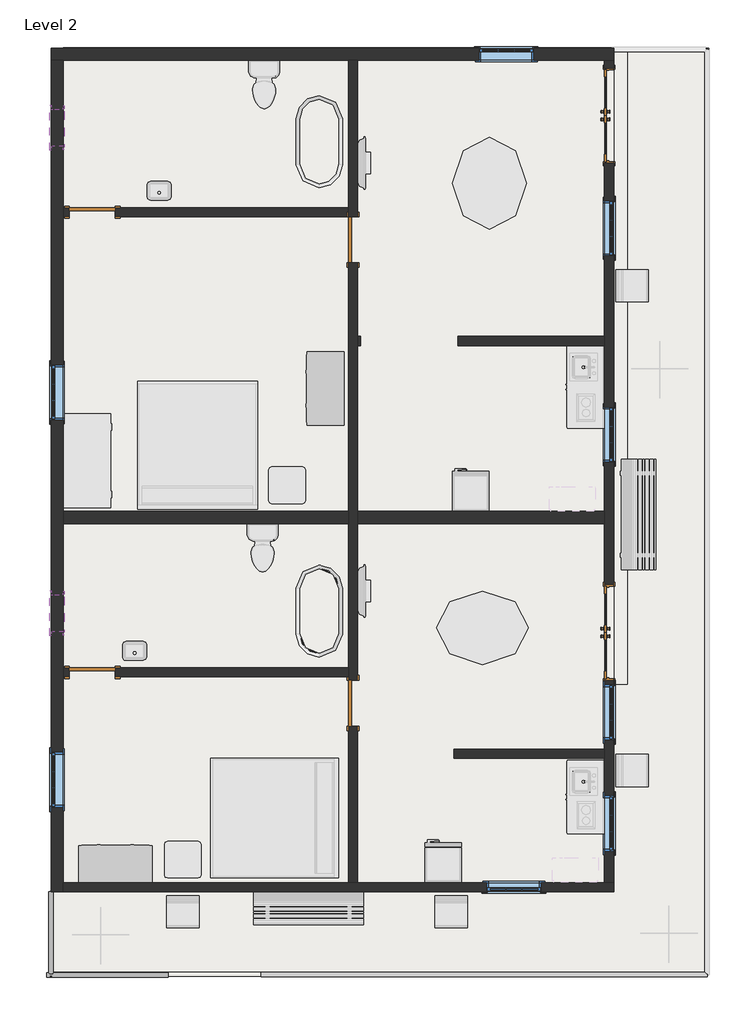
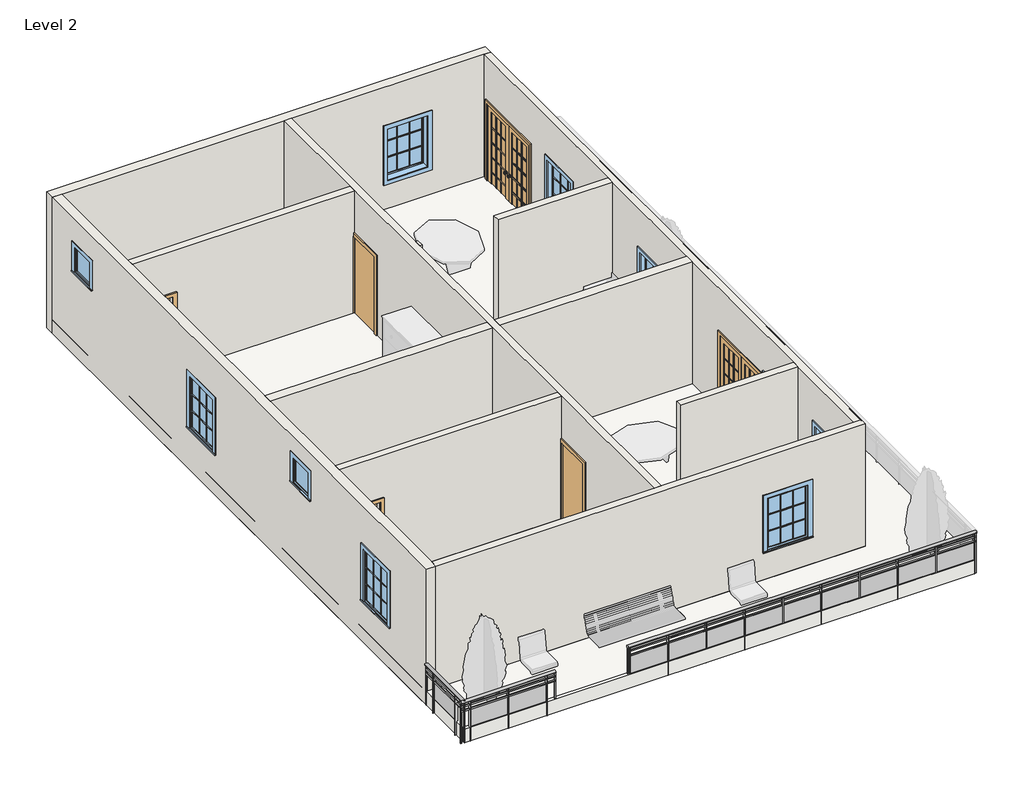
# One storey, part 1 of 2: 12 walls, 10 windows, 7 roofs, 6 doors, 3 railings.
"""IFC4 building model written with IfcOpenShell, lengths in millimetres."""

from ifc_helpers import new_model, si_unit, point, frame, origin, place, context, project, spatial, polyline, ellipse_curve, trimmed, outline, extrude, faceted_brep, transform, mapped, element, save
from ifc_brep_helpers import plane_surface, extruded_surface, advanced_brep
from components import door_31a77bde, door_255cab33, door_059fdd7e, window_29c06734, window_5c190c7e, window_e41d21a6

model = new_model("IFC4")

# Units and contexts
model_context = context("Model", 3, world=origin())
ifc_project = project(units=[si_unit("LENGTHUNIT", "METRE", prefix="MILLI")], contexts=[model_context])

# Site, building, storey
site = spatial("IfcSite", under=ifc_project)
building = spatial("IfcBuilding", under=site)
storey = spatial("IfcBuildingStorey", under=building, Name="Level 2", Elevation=3048.0)

# Doors
placement = place(None, origin())
door_shape = door_31a77bde(model_context)
element("IfcDoor", 1, ObjectType="Door-Interior-Double-Full Glass-Wood : 60\" x 80\"", at=placement, inside=storey, context=model_context, shape_type="MappedRepresentation", body=[
    mapped(door_shape, transform((230.0079734, 3216.1923354, 3048.0), x_axis=(0.0, 1.0, 0.0), y_axis=(-1.0, 0.0, 0.0), z_axis=(0.0, 0.0, 1.0))),
])
element("IfcDoor", 2, ObjectType="Door-Interior-Double-Full Glass-Wood : 60\" x 80\"", at=placement, inside=storey, context=model_context, shape_type="MappedRepresentation", body=[
    mapped(door_shape, transform((230.0079734, 11775.9923354, 3048.0), x_axis=(0.0, 1.0, 0.0), y_axis=(-1.0, 0.0, 0.0), z_axis=(0.0, 0.0, 1.0))),
])
door_2_shape = door_255cab33(model_context)
element("IfcDoor", 3, ObjectType="Single-Flush : 30\" x 80\"", at=placement, inside=storey, context=model_context, shape_type="MappedRepresentation", body=[
    mapped(door_2_shape, transform((-8326.6170266, 10175.7923354, 3048.0), x_axis=(-1.0, 0.0, 0.0), y_axis=(0.0, -1.0, 0.0), z_axis=(0.0, 0.0, 1.0))),
])
element("IfcDoor", 4, ObjectType="Single-Flush : 30\" x 80\"", at=placement, inside=storey, context=model_context, shape_type="MappedRepresentation", body=[
    mapped(door_2_shape, transform((-8326.6170266, 2555.7923354, 3048.0), x_axis=(-1.0, 0.0, 0.0), y_axis=(0.0, -1.0, 0.0), z_axis=(0.0, 0.0, 1.0))),
])
door_3_shape = door_059fdd7e(model_context)
element("IfcDoor", 5, ObjectType="Single-Flush : 30\" x 80\"", at=placement, inside=storey, context=model_context, shape_type="MappedRepresentation", body=[
    mapped(door_3_shape, transform((-4008.6170266, 9718.5923354, 3048.0), x_axis=(0.0, 1.0, 0.0), y_axis=(-1.0, 0.0, 0.0), z_axis=(0.0, 0.0, 1.0))),
])
element("IfcDoor", 6, ObjectType="Single-Flush : 30\" x 80\"", at=placement, inside=storey, context=model_context, shape_type="MappedRepresentation", body=[
    mapped(door_3_shape, transform((-4008.6170266, 2047.7923354, 3048.0), x_axis=(0.0, 1.0, 0.0), y_axis=(-1.0, 0.0, 0.0), z_axis=(0.0, 0.0, 1.0))),
])

# Railings
element("IfcRailing", 7, ObjectType="Glass Panel - Bottom Fill", at=placement, inside=storey, context=model_context, shape_type="SolidModel", body=[
    advanced_brep(
    [(-8974.3170266, -1076.4076646, 3962.4), (-9050.5170266, -1076.4076646, 3962.4), (-8974.3170266, -2473.4076646, 3962.4), (-9050.5170266, -2473.4076646, 3962.4)],
    [
        (0, 1, ellipse_curve(frame((-9012.4170266, -1076.4076646, 3962.4), z_axis=(0.0, 1.0, 0.0), x_axis=(-1.0, 0.0, 0.0)), 38.1, 28.575)),
        (1, 0, ellipse_curve(frame((-9012.4170266, -1076.4076646, 3962.4), z_axis=(0.0, 1.0, 0.0), x_axis=(-1.0, 0.0, 0.0)), 38.1, 28.575)),
        (2, 3, ellipse_curve(frame((-9012.4170266, -2473.4076646, 3962.4), z_axis=(0.0, -1.0, 0.0), x_axis=(-1.0, 0.0, 0.0)), 38.1, 28.575)),
        (3, 2, ellipse_curve(frame((-9012.4170266, -2473.4076646, 3962.4), z_axis=(0.0, -1.0, 0.0), x_axis=(-1.0, 0.0, 0.0)), 38.1, 28.575)),
        (0, 2),
        (3, 1),
    ],
    [
        plane_surface(frame((-9012.4170266, -1076.4076646, 3962.4), z_axis=(0.0, 1.0, 0.0), x_axis=(0.0, 0.0, -1.0))),
        plane_surface(frame((-9012.4170266, -2473.4076646, 3962.4), z_axis=(0.0, -1.0, 0.0), x_axis=(0.0, 0.0, -1.0))),
        extruded_surface(trimmed(ellipse_curve(frame((-9012.4170266, -2473.4076646, 3962.4), z_axis=(0.0, 1.0, 0.0), x_axis=(-1.0, 0.0, 0.0)), 38.1, 28.575), [point((-8974.3170266, -2473.4076646, 3962.4))], [point((-9050.5170266, -2473.4076646, 3962.4))], True, "CARTESIAN"), (0.0, 1396.9999999999998, 0.0), 1396.9999999999998),
        extruded_surface(trimmed(ellipse_curve(frame((-9012.4170266, -2473.4076646, 3962.4), z_axis=(0.0, 1.0, 0.0), x_axis=(-1.0, 0.0, 0.0)), 38.1, 28.575), [point((-9050.5170266, -2473.4076646, 3962.4))], [point((-8974.3170266, -2473.4076646, 3962.4))], True, "CARTESIAN"), (0.0, 1396.9999999999998, 0.0), 1396.9999999999998),
    ],
    [
        (0, [[1, 2]]),
        (1, [[3, 4]]),
        (2, [[-1, 5, -4, 6]]),
        (3, [[-2, -6, -3, -5]]),
    ],
),
    extrude(outline(polyline([(-9025.1170266, -1076.4076646), (-8999.7170266, -1076.4076646), (-8999.7170266, -2473.4076646), (-9025.1170266, -2473.4076646), (-9025.1170266, -1076.4076646)])), frame((0.0, 0.0, 3848.1), z_axis=(0.0, 0.0, 1.0), x_axis=(1.0, 0.0, 0.0)), (0.0, 0.0, 1.0), 25.4),
    extrude(outline(polyline([(-9025.1170266, -1076.4076646), (-8999.7170266, -1076.4076646), (-8999.7170266, -2473.4076646), (-9025.1170266, -2473.4076646), (-9025.1170266, -1076.4076646)])), frame((0.0, 0.0, 3746.5), z_axis=(0.0, 0.0, 1.0), x_axis=(1.0, 0.0, 0.0)), (0.0, 0.0, 1.0), 25.4),
    extrude(outline(polyline([(-9037.8170266, -2174.9576646), (-8987.0170266, -2174.9576646), (-8987.0170266, -2187.6576646), (-9037.8170266, -2187.6576646), (-9037.8170266, -2174.9576646)])), frame((0.0, 0.0, 3048.0), z_axis=(0.0, 0.0, 1.0), x_axis=(1.0, 0.0, 0.0)), (0.0, 0.0, 1.0), 885.6788223),
    extrude(outline(polyline([(-9005.8818696, -1368.5076646), (-9005.8818696, -2181.3076646), (-9012.2318696, -2181.3076646), (-9012.2318696, -1368.5076646), (-9005.8818696, -1368.5076646)])), frame((0.0, 0.0, 3149.6), z_axis=(0.0, 0.0, 1.0), x_axis=(1.0, 0.0, 0.0)), (0.0, 0.0, 1.0), 596.9),
    extrude(outline(polyline([(-9037.8170266, -1362.1576646), (-8987.0170266, -1362.1576646), (-8987.0170266, -1374.8576646), (-9037.8170266, -1374.8576646), (-9037.8170266, -1362.1576646)])), frame((0.0, 0.0, 3048.0), z_axis=(0.0, 0.0, 1.0), x_axis=(1.0, 0.0, 0.0)), (0.0, 0.0, 1.0), 885.6788223),
    extrude(outline(polyline([(-9021.9420266, -2460.7076646), (-9002.8920266, -2460.7076646), (-9002.8920266, -2479.7576646), (-9021.9420266, -2479.7576646), (-9021.9420266, -2460.7076646)])), frame((0.0, 0.0, 3048.0), z_axis=(0.0, 0.0, 1.0), x_axis=(1.0, 0.0, 0.0)), (0.0, 0.0, 1.0), 885.6788223),
    extrude(outline(polyline([(-9021.9420266, -1070.0576646), (-9002.8920266, -1070.0576646), (-9002.8920266, -1089.1076646), (-9021.9420266, -1089.1076646), (-9021.9420266, -1070.0576646)])), frame((0.0, 0.0, 3048.0), z_axis=(0.0, 0.0, 1.0), x_axis=(1.0, 0.0, 0.0)), (0.0, 0.0, 1.0), 885.6788223),
])
element("IfcRailing", 8, ObjectType="Glass Panel - Bottom Fill", at=placement, inside=storey, context=model_context, shape_type="SolidModel", body=[
    advanced_brep(
    [(-9080.8545291, -2419.5212738, 3962.4), (-9080.8545291, -2495.7212738, 3962.4), (-7074.2545291, -2419.5212738, 3962.4), (-7074.2545291, -2495.7212738, 3962.4)],
    [
        (0, 1, ellipse_curve(frame((-9080.8545291, -2457.6212738, 3962.4), z_axis=(-1.0, 0.0, 0.0), x_axis=(0.0, -1.0, 0.0)), 38.1, 28.575)),
        (1, 0, ellipse_curve(frame((-9080.8545291, -2457.6212738, 3962.4), z_axis=(-1.0, 0.0, 0.0), x_axis=(0.0, -1.0, 0.0)), 38.1, 28.575)),
        (2, 3, ellipse_curve(frame((-7074.2545291, -2457.6212738, 3962.4), z_axis=(1.0, 0.0, 0.0), x_axis=(0.0, -1.0, 0.0)), 38.1, 28.575)),
        (3, 2, ellipse_curve(frame((-7074.2545291, -2457.6212738, 3962.4), z_axis=(1.0, 0.0, 0.0), x_axis=(0.0, -1.0, 0.0)), 38.1, 28.575)),
        (0, 2),
        (3, 1),
    ],
    [
        plane_surface(frame((-9080.8545291, -2457.6212738, 3962.4), z_axis=(-1.0, 0.0, 0.0), x_axis=(0.0, 1.0, 0.0))),
        plane_surface(frame((-7074.2545291, -2457.6212738, 3962.4), z_axis=(1.0, 0.0, 0.0), x_axis=(0.0, 1.0, 0.0))),
        extruded_surface(trimmed(ellipse_curve(frame((-7074.2545291, -2457.6212738, 3962.4), z_axis=(-1.0, 0.0, 0.0), x_axis=(0.0, -1.0, 0.0)), 38.1, 28.575), [point((-7074.2545291, -2419.5212738, 3962.4))], [point((-7074.2545291, -2495.7212738, 3962.4))], True, "CARTESIAN"), (-2006.5999999999995, 0.0, 0.0), 2006.5999999999995),
        extruded_surface(trimmed(ellipse_curve(frame((-7074.2545291, -2457.6212738, 3962.4), z_axis=(-1.0, 0.0, 0.0), x_axis=(0.0, -1.0, 0.0)), 38.1, 28.575), [point((-7074.2545291, -2495.7212738, 3962.4))], [point((-7074.2545291, -2419.5212738, 3962.4))], True, "CARTESIAN"), (-2006.5999999999995, 0.0, 0.0), 2006.5999999999995),
    ],
    [
        (0, [[1, 2]]),
        (1, [[3, 4]]),
        (2, [[-1, 5, -4, 6]]),
        (3, [[-2, -6, -3, -5]]),
    ],
),
    extrude(outline(polyline([(-9080.8545291, -2470.3212738), (-9080.8545291, -2444.9212738), (-7074.2545291, -2444.9212738), (-7074.2545291, -2470.3212738), (-9080.8545291, -2470.3212738)])), frame((0.0, 0.0, 3848.1), z_axis=(0.0, 0.0, 1.0), x_axis=(1.0, 0.0, 0.0)), (0.0, 0.0, 1.0), 25.4),
    extrude(outline(polyline([(-9080.8545291, -2470.3212738), (-9080.8545291, -2444.9212738), (-7074.2545291, -2444.9212738), (-7074.2545291, -2470.3212738), (-9080.8545291, -2470.3212738)])), frame((0.0, 0.0, 3746.5), z_axis=(0.0, 0.0, 1.0), x_axis=(1.0, 0.0, 0.0)), (0.0, 0.0, 1.0), 25.4),
    extrude(outline(polyline([(-7271.1045291, -2483.0212738), (-7271.1045291, -2432.2212738), (-7258.4045291, -2432.2212738), (-7258.4045291, -2483.0212738), (-7271.1045291, -2483.0212738)])), frame((0.0, 0.0, 3048.0), z_axis=(0.0, 0.0, 1.0), x_axis=(1.0, 0.0, 0.0)), (0.0, 0.0, 1.0), 885.6788223),
    extrude(outline(polyline([(-8077.5545291, -2451.0861168), (-7264.7545291, -2451.0861168), (-7264.7545291, -2457.4361168), (-8077.5545291, -2457.4361168), (-8077.5545291, -2451.0861168)])), frame((0.0, 0.0, 3149.6), z_axis=(0.0, 0.0, 1.0), x_axis=(1.0, 0.0, 0.0)), (0.0, 0.0, 1.0), 596.9),
    extrude(outline(polyline([(-8083.9045291, -2483.0212738), (-8083.9045291, -2432.2212738), (-8071.2045291, -2432.2212738), (-8071.2045291, -2483.0212738), (-8083.9045291, -2483.0212738)])), frame((0.0, 0.0, 3048.0), z_axis=(0.0, 0.0, 1.0), x_axis=(1.0, 0.0, 0.0)), (0.0, 0.0, 1.0), 885.6788223),
    extrude(outline(polyline([(-8890.3545291, -2451.0861168), (-8077.5545291, -2451.0861168), (-8077.5545291, -2457.4361168), (-8890.3545291, -2457.4361168), (-8890.3545291, -2451.0861168)])), frame((0.0, 0.0, 3149.6), z_axis=(0.0, 0.0, 1.0), x_axis=(1.0, 0.0, 0.0)), (0.0, 0.0, 1.0), 596.9),
    extrude(outline(polyline([(-8896.7045291, -2483.0212738), (-8896.7045291, -2432.2212738), (-8884.0045291, -2432.2212738), (-8884.0045291, -2483.0212738), (-8896.7045291, -2483.0212738)])), frame((0.0, 0.0, 3048.0), z_axis=(0.0, 0.0, 1.0), x_axis=(1.0, 0.0, 0.0)), (0.0, 0.0, 1.0), 885.6788223),
    extrude(outline(polyline([(-7086.9545291, -2467.1462738), (-7086.9545291, -2448.0962738), (-7067.9045291, -2448.0962738), (-7067.9045291, -2467.1462738), (-7086.9545291, -2467.1462738)])), frame((0.0, 0.0, 3048.0), z_axis=(0.0, 0.0, 1.0), x_axis=(1.0, 0.0, 0.0)), (0.0, 0.0, 1.0), 885.6788223),
    extrude(outline(polyline([(-9087.2045291, -2467.1462738), (-9087.2045291, -2448.0962738), (-9068.1545291, -2448.0962738), (-9068.1545291, -2467.1462738), (-9087.2045291, -2467.1462738)])), frame((0.0, 0.0, 3048.0), z_axis=(0.0, 0.0, 1.0), x_axis=(1.0, 0.0, 0.0)), (0.0, 0.0, 1.0), 885.6788223),
])
element("IfcRailing", 9, ObjectType="Glass Panel - Bottom Fill", at=placement, inside=storey, context=model_context, shape_type="SolidModel", body=[
    advanced_brep(
    [(1862.5146653, -2486.1076646, 3962.4), (1862.5146653, -2409.9076646, 3962.4), (-5528.8853347, -2486.1076646, 3962.4), (-5528.8853347, -2409.9076646, 3962.4)],
    [
        (0, 1, ellipse_curve(frame((1862.5146653, -2448.0076646, 3962.4), z_axis=(1.0, 0.0, 0.0), x_axis=(0.0, 1.0, 0.0)), 38.1, 28.575)),
        (1, 0, ellipse_curve(frame((1862.5146653, -2448.0076646, 3962.4), z_axis=(1.0, 0.0, 0.0), x_axis=(0.0, 1.0, 0.0)), 38.1, 28.575)),
        (2, 3, ellipse_curve(frame((-5528.8853347, -2448.0076646, 3962.4), z_axis=(-1.0, 0.0, 0.0), x_axis=(0.0, 1.0, 0.0)), 38.1, 28.575)),
        (3, 2, ellipse_curve(frame((-5528.8853347, -2448.0076646, 3962.4), z_axis=(-1.0, 0.0, 0.0), x_axis=(0.0, 1.0, 0.0)), 38.1, 28.575)),
        (0, 2),
        (3, 1),
    ],
    [
        plane_surface(frame((1862.5146653, -2448.0076646, 3962.4), z_axis=(1.0, 0.0, 0.0), x_axis=(0.0, -1.0, 0.0))),
        plane_surface(frame((-5528.8853347, -2448.0076646, 3962.4), z_axis=(-1.0, 0.0, 0.0), x_axis=(0.0, -1.0, 0.0))),
        extruded_surface(trimmed(ellipse_curve(frame((-5528.8853347, -2448.0076646, 3962.4), z_axis=(1.0, 0.0, 0.0), x_axis=(0.0, 1.0, 0.0)), 38.1, 28.575), [point((-5528.8853347, -2486.1076646, 3962.4))], [point((-5528.8853347, -2409.9076646, 3962.4))], True, "CARTESIAN"), (7391.400000000001, 0.0, 0.0), 7391.400000000001),
        extruded_surface(trimmed(ellipse_curve(frame((-5528.8853347, -2448.0076646, 3962.4), z_axis=(1.0, 0.0, 0.0), x_axis=(0.0, 1.0, 0.0)), 38.1, 28.575), [point((-5528.8853347, -2409.9076646, 3962.4))], [point((-5528.8853347, -2486.1076646, 3962.4))], True, "CARTESIAN"), (7391.400000000001, 0.0, 0.0), 7391.400000000001),
    ],
    [
        (0, [[1, 2]]),
        (1, [[3, 4]]),
        (2, [[-1, 5, -4, 6]]),
        (3, [[-2, -6, -3, -5]]),
    ],
),
    extrude(outline(polyline([(1862.5146653, -2435.3076646), (1862.5146653, -2460.7076646), (-5528.8853347, -2460.7076646), (-5528.8853347, -2435.3076646), (1862.5146653, -2435.3076646)])), frame((0.0, 0.0, 3848.1), z_axis=(0.0, 0.0, 1.0), x_axis=(1.0, 0.0, 0.0)), (0.0, 0.0, 1.0), 25.4),
    extrude(outline(polyline([(1862.5146653, -2435.3076646), (1862.5146653, -2460.7076646), (-5528.8853347, -2460.7076646), (-5528.8853347, -2435.3076646), (1862.5146653, -2435.3076646)])), frame((0.0, 0.0, 3746.5), z_axis=(0.0, 0.0, 1.0), x_axis=(1.0, 0.0, 0.0)), (0.0, 0.0, 1.0), 25.4),
    extrude(outline(polyline([(-5484.4353347, -2422.6076646), (-5484.4353347, -2473.4076646), (-5497.1353347, -2473.4076646), (-5497.1353347, -2422.6076646), (-5484.4353347, -2422.6076646)])), frame((0.0, 0.0, 3048.0), z_axis=(0.0, 0.0, 1.0), x_axis=(1.0, 0.0, 0.0)), (0.0, 0.0, 1.0), 885.6788223),
    extrude(outline(polyline([(-4677.9853347, -2454.5428216), (-5490.7853347, -2454.5428216), (-5490.7853347, -2448.1928216), (-4677.9853347, -2448.1928216), (-4677.9853347, -2454.5428216)])), frame((0.0, 0.0, 3149.6), z_axis=(0.0, 0.0, 1.0), x_axis=(1.0, 0.0, 0.0)), (0.0, 0.0, 1.0), 596.9),
    extrude(outline(polyline([(-4671.6353347, -2422.6076646), (-4671.6353347, -2473.4076646), (-4684.3353347, -2473.4076646), (-4684.3353347, -2422.6076646), (-4671.6353347, -2422.6076646)])), frame((0.0, 0.0, 3048.0), z_axis=(0.0, 0.0, 1.0), x_axis=(1.0, 0.0, 0.0)), (0.0, 0.0, 1.0), 885.6788223),
    extrude(outline(polyline([(-3865.1853347, -2454.5428216), (-4677.9853347, -2454.5428216), (-4677.9853347, -2448.1928216), (-3865.1853347, -2448.1928216), (-3865.1853347, -2454.5428216)])), frame((0.0, 0.0, 3149.6), z_axis=(0.0, 0.0, 1.0), x_axis=(1.0, 0.0, 0.0)), (0.0, 0.0, 1.0), 596.9),
    extrude(outline(polyline([(-3858.8353347, -2422.6076646), (-3858.8353347, -2473.4076646), (-3871.5353347, -2473.4076646), (-3871.5353347, -2422.6076646), (-3858.8353347, -2422.6076646)])), frame((0.0, 0.0, 3048.0), z_axis=(0.0, 0.0, 1.0), x_axis=(1.0, 0.0, 0.0)), (0.0, 0.0, 1.0), 885.6788223),
    extrude(outline(polyline([(-3052.3853347, -2454.5428216), (-3865.1853347, -2454.5428216), (-3865.1853347, -2448.1928216), (-3052.3853347, -2448.1928216), (-3052.3853347, -2454.5428216)])), frame((0.0, 0.0, 3149.6), z_axis=(0.0, 0.0, 1.0), x_axis=(1.0, 0.0, 0.0)), (0.0, 0.0, 1.0), 596.9),
    extrude(outline(polyline([(-3046.0353347, -2422.6076646), (-3046.0353347, -2473.4076646), (-3058.7353347, -2473.4076646), (-3058.7353347, -2422.6076646), (-3046.0353347, -2422.6076646)])), frame((0.0, 0.0, 3048.0), z_axis=(0.0, 0.0, 1.0), x_axis=(1.0, 0.0, 0.0)), (0.0, 0.0, 1.0), 885.6788223),
    extrude(outline(polyline([(-2239.5853347, -2454.5428216), (-3052.3853347, -2454.5428216), (-3052.3853347, -2448.1928216), (-2239.5853347, -2448.1928216), (-2239.5853347, -2454.5428216)])), frame((0.0, 0.0, 3149.6), z_axis=(0.0, 0.0, 1.0), x_axis=(1.0, 0.0, 0.0)), (0.0, 0.0, 1.0), 596.9),
    extrude(outline(polyline([(-2233.2353347, -2422.6076646), (-2233.2353347, -2473.4076646), (-2245.9353347, -2473.4076646), (-2245.9353347, -2422.6076646), (-2233.2353347, -2422.6076646)])), frame((0.0, 0.0, 3048.0), z_axis=(0.0, 0.0, 1.0), x_axis=(1.0, 0.0, 0.0)), (0.0, 0.0, 1.0), 885.6788223),
    extrude(outline(polyline([(-1426.7853347, -2454.5428216), (-2239.5853347, -2454.5428216), (-2239.5853347, -2448.1928216), (-1426.7853347, -2448.1928216), (-1426.7853347, -2454.5428216)])), frame((0.0, 0.0, 3149.6), z_axis=(0.0, 0.0, 1.0), x_axis=(1.0, 0.0, 0.0)), (0.0, 0.0, 1.0), 596.9),
    extrude(outline(polyline([(-1420.4353347, -2422.6076646), (-1420.4353347, -2473.4076646), (-1433.1353347, -2473.4076646), (-1433.1353347, -2422.6076646), (-1420.4353347, -2422.6076646)])), frame((0.0, 0.0, 3048.0), z_axis=(0.0, 0.0, 1.0), x_axis=(1.0, 0.0, 0.0)), (0.0, 0.0, 1.0), 885.6788223),
    extrude(outline(polyline([(-613.9853347, -2454.5428216), (-1426.7853347, -2454.5428216), (-1426.7853347, -2448.1928216), (-613.9853347, -2448.1928216), (-613.9853347, -2454.5428216)])), frame((0.0, 0.0, 3149.6), z_axis=(0.0, 0.0, 1.0), x_axis=(1.0, 0.0, 0.0)), (0.0, 0.0, 1.0), 596.9),
    extrude(outline(polyline([(-607.6353347, -2422.6076646), (-607.6353347, -2473.4076646), (-620.3353347, -2473.4076646), (-620.3353347, -2422.6076646), (-607.6353347, -2422.6076646)])), frame((0.0, 0.0, 3048.0), z_axis=(0.0, 0.0, 1.0), x_axis=(1.0, 0.0, 0.0)), (0.0, 0.0, 1.0), 885.6788223),
    extrude(outline(polyline([(198.8146653, -2454.5428216), (-613.9853347, -2454.5428216), (-613.9853347, -2448.1928216), (198.8146653, -2448.1928216), (198.8146653, -2454.5428216)])), frame((0.0, 0.0, 3149.6), z_axis=(0.0, 0.0, 1.0), x_axis=(1.0, 0.0, 0.0)), (0.0, 0.0, 1.0), 596.9),
    extrude(outline(polyline([(205.1646653, -2422.6076646), (205.1646653, -2473.4076646), (192.4646653, -2473.4076646), (192.4646653, -2422.6076646), (205.1646653, -2422.6076646)])), frame((0.0, 0.0, 3048.0), z_axis=(0.0, 0.0, 1.0), x_axis=(1.0, 0.0, 0.0)), (0.0, 0.0, 1.0), 885.6788223),
    extrude(outline(polyline([(1011.6146653, -2454.5428216), (198.8146653, -2454.5428216), (198.8146653, -2448.1928216), (1011.6146653, -2448.1928216), (1011.6146653, -2454.5428216)])), frame((0.0, 0.0, 3149.6), z_axis=(0.0, 0.0, 1.0), x_axis=(1.0, 0.0, 0.0)), (0.0, 0.0, 1.0), 596.9),
    extrude(outline(polyline([(1017.9646653, -2422.6076646), (1017.9646653, -2473.4076646), (1005.2646653, -2473.4076646), (1005.2646653, -2422.6076646), (1017.9646653, -2422.6076646)])), frame((0.0, 0.0, 3048.0), z_axis=(0.0, 0.0, 1.0), x_axis=(1.0, 0.0, 0.0)), (0.0, 0.0, 1.0), 885.6788223),
    extrude(outline(polyline([(1824.4146653, -2454.5428216), (1011.6146653, -2454.5428216), (1011.6146653, -2448.1928216), (1824.4146653, -2448.1928216), (1824.4146653, -2454.5428216)])), frame((0.0, 0.0, 3149.6), z_axis=(0.0, 0.0, 1.0), x_axis=(1.0, 0.0, 0.0)), (0.0, 0.0, 1.0), 596.9),
    extrude(outline(polyline([(1830.7646653, -2422.6076646), (1830.7646653, -2473.4076646), (1818.0646653, -2473.4076646), (1818.0646653, -2422.6076646), (1830.7646653, -2422.6076646)])), frame((0.0, 0.0, 3048.0), z_axis=(0.0, 0.0, 1.0), x_axis=(1.0, 0.0, 0.0)), (0.0, 0.0, 1.0), 885.6788223),
    extrude(outline(polyline([(-5516.1853347, -2438.4826646), (-5516.1853347, -2457.5326646), (-5535.2353347, -2457.5326646), (-5535.2353347, -2438.4826646), (-5516.1853347, -2438.4826646)])), frame((0.0, 0.0, 3048.0), z_axis=(0.0, 0.0, 1.0), x_axis=(1.0, 0.0, 0.0)), (0.0, 0.0, 1.0), 885.6788223),
    extrude(outline(polyline([(1868.8646653, -2438.4826646), (1868.8646653, -2457.5326646), (1849.8146653, -2457.5326646), (1849.8146653, -2438.4826646), (1868.8646653, -2438.4826646)])), frame((0.0, 0.0, 3048.0), z_axis=(0.0, 0.0, 1.0), x_axis=(1.0, 0.0, 0.0)), (0.0, 0.0, 1.0), 885.6788223),
])

# Roofs
element("IfcRoof", 10, ObjectType="Generic - 12\"", at=placement, inside=storey, context=model_context, shape_type="SweptSolid", body=[
    extrude(outline(polyline([(-9012.4170266, 12893.5923354), (1858.7829734, 12893.5923354), (1858.7829734, -2397.2076646), (-9012.4170266, -2397.2076646), (-9012.4170266, 12893.5923354)])), frame((0.0, 0.0, 3048.0), z_axis=(0.0, 0.0, 1.0), x_axis=(1.0, 0.0, 0.0)), (0.0, 0.0, 1.0), 304.8),
])
element("IfcRoof", 11, ObjectType="Generic - 12\"", at=placement, inside=storey, context=model_context, shape_type="SweptSolid", body=[
    extrude(outline(polyline([(-9012.4170266, 12893.5923354), (1818.7665921, 12893.5923354), (1818.7665921, -2473.4076646), (-9012.4170266, -2473.4076646), (-9012.4170266, 12893.5923354)])), frame((0.0, 0.0, 3048.0), z_axis=(0.0, 0.0, 1.0), x_axis=(1.0, 0.0, 0.0)), (0.0, 0.0, 1.0), 304.8),
])
element("IfcRoof", 12, ObjectType="Generic - 12\"", at=placement, inside=storey, context=model_context, shape_type="SweptSolid", body=[
    extrude(outline(polyline([(-8809.2170266, 12690.3923354), (309.3829734, 12690.3923354), (309.3829734, -1076.4076646), (-8809.2170266, -1076.4076646), (-8809.2170266, 12690.3923354)])), frame((0.0, 0.0, 3048.0), z_axis=(0.0, 0.0, 1.0), x_axis=(1.0, 0.0, 0.0)), (0.0, 0.0, 1.0), 304.8),
])
element("IfcRoof", 13, ObjectType="Generic - 12\"", at=placement, inside=storey, context=model_context, shape_type="SweptSolid", body=[
    extrude(outline(polyline([(-8809.2170266, 12690.3923354), (309.3829734, 12690.3923354), (309.3829734, -1076.4076646), (-8809.2170266, -1076.4076646), (-8809.2170266, 12690.3923354)])), frame((0.0, 0.0, 3048.0), z_axis=(0.0, 0.0, 1.0), x_axis=(1.0, 0.0, 0.0)), (0.0, 0.0, 1.0), 304.8),
])
element("IfcRoof", 14, ObjectType="Generic - 12\"", at=placement, inside=storey, context=model_context, shape_type="SweptSolid", body=[
    extrude(outline(polyline([(-8809.2170266, 12899.4292281), (537.9829734, 12899.4292281), (537.9829734, 2358.4292281), (-8809.2170266, 2358.4292281), (-8809.2170266, 12899.4292281)])), frame((0.0, 0.0, 3048.0), z_axis=(0.0, 0.0, 1.0), x_axis=(1.0, 0.0, 0.0)), (0.0, 0.0, 1.0), 304.8),
])
element("IfcRoof", 15, ObjectType="Generic - 12\"", at=placement, inside=storey, context=model_context, shape_type="SweptSolid", body=[
    extrude(outline(polyline([(-9012.4170266, 12893.5923354), (1884.1829734, 12893.5923354), (1884.1829734, 5203.7423354), (-9012.4170266, 5203.7423354), (-9012.4170266, 12893.5923354)])), frame((0.0, 0.0, 3048.0), z_axis=(0.0, 0.0, 1.0), x_axis=(1.0, 0.0, 0.0)), (0.0, 0.0, 1.0), 304.8),
])
element("IfcRoof", 16, ObjectType="Generic - 12\"", at=placement, inside=storey, context=model_context, shape_type="SweptSolid", body=[
    extrude(outline(polyline([(-9012.4170266, 12893.5923354), (1858.7829734, 12893.5923354), (1858.7829734, -2397.2076646), (-9012.4170266, -2397.2076646), (-9012.4170266, 12893.5923354)])), frame((0.0, 0.0, 3048.0), z_axis=(0.0, 0.0, 1.0), x_axis=(1.0, 0.0, 0.0)), (0.0, 0.0, 1.0), 304.8),
])

# Walls
element("IfcWall", 17, ObjectType="Generic - 8\"", at=placement, inside=storey, context=model_context, shape_type="Brep", body=[
    faceted_brep([(-9012.4170266, 12690.3923354, 3048.0), (-8809.2170266, 12690.3923354, 3048.0), (-4084.8170266, 12690.3923354, 3048.0), (-3932.4170266, 12690.3923354, 3048.0), (156.9829734, 12690.3923354, 3048.0), (309.3829734, 12690.3923354, 3048.0), (309.3829734, 12690.3923354, 6096.0), (156.9829734, 12690.3923354, 6096.0), (-3932.4170266, 12690.3923354, 6096.0), (-4084.8170266, 12690.3923354, 6096.0), (-8809.2170266, 12690.3923354, 6096.0), (-9012.4170266, 12690.3923354, 6096.0), (-1011.4170266, 12690.3923354, 5181.6), (-1011.4170266, 12690.3923354, 3962.4), (-1925.8170266, 12690.3923354, 3962.4), (-1925.8170266, 12690.3923354, 5181.6), (-9012.4170266, 12893.5923354, 3048.0), (-9012.4170266, 12893.5923354, 6096.0), (309.3829734, 12893.5923354, 6096.0), (309.3829734, 12893.5923354, 3048.0), (-1011.4170266, 12893.5923354, 5181.6), (-1925.8170266, 12893.5923354, 5181.6), (-1925.8170266, 12893.5923354, 3962.4), (-1011.4170266, 12893.5923354, 3962.4)], [[[0, 1, 2, 3, 4, 5, 6, 7, 8, 9, 10, 11], [12, 13, 14, 15]], [[16, 17, 18, 19], [20, 21, 22, 23]], [[5, 4, 3, 2, 1, 0, 16, 19]], [[11, 10, 9, 8, 7, 6, 18, 17]], [[0, 11, 17, 16]], [[6, 5, 19, 18]], [[13, 12, 20, 23]], [[14, 13, 23, 22]], [[15, 14, 22, 21]], [[12, 15, 21, 20]]]),
])
element("IfcWall", 18, ObjectType="Generic - 8\"", at=placement, inside=storey, context=model_context, shape_type="Brep", body=[
    faceted_brep([(-8809.2170266, -1076.4076646, 3048.0), (-8809.2170266, -924.0076646, 3048.0), (-8809.2170266, 2479.5923354, 3048.0), (-8809.2170266, 2631.9923354, 3048.0), (-8809.2170266, 5019.5923354, 3048.0), (-8809.2170266, 5222.7923354, 3048.0), (-8809.2170266, 10099.5923354, 3048.0), (-8809.2170266, 10251.9923354, 3048.0), (-8809.2170266, 12690.3923354, 3048.0), (-8809.2170266, 12690.3923354, 6096.0), (-8809.2170266, 10251.9923354, 6096.0), (-8809.2170266, 10099.5923354, 6096.0), (-8809.2170266, 5222.7923354, 6096.0), (-8809.2170266, 5019.5923354, 6096.0), (-8809.2170266, 2631.9923354, 6096.0), (-8809.2170266, 2479.5923354, 6096.0), (-8809.2170266, -924.0076646, 6096.0), (-8809.2170266, -1076.4076646, 6096.0), (-8809.2170266, 11877.5923354, 5511.8), (-8809.2170266, 11877.5923354, 4902.2), (-8809.2170266, 11267.9923354, 4902.2), (-8809.2170266, 11267.9923354, 5511.8), (-8809.2170266, 3838.4923354, 5664.2), (-8809.2170266, 3838.4923354, 5054.6), (-8809.2170266, 3228.8923354, 5054.6), (-8809.2170266, 3228.8923354, 5664.2), (-8809.2170266, 7648.4923354, 5181.6), (-8809.2170266, 7648.4923354, 3962.4), (-8809.2170266, 6734.0923354, 3962.4), (-8809.2170266, 6734.0923354, 5181.6), (-8809.2170266, 1234.9923354, 5181.6), (-8809.2170266, 1234.9923354, 3962.4), (-8809.2170266, 320.5923354, 3962.4), (-8809.2170266, 320.5923354, 5181.6), (-9012.4170266, -1076.4076646, 3048.0), (-9012.4170266, -1076.4076646, 6096.0), (-9012.4170266, 12690.3923354, 6096.0), (-9012.4170266, 12690.3923354, 3048.0), (-9012.4170266, 11877.5923354, 5511.8), (-9012.4170266, 11267.9923354, 5511.8), (-9012.4170266, 11267.9923354, 4902.2), (-9012.4170266, 11877.5923354, 4902.2), (-9012.4170266, 3838.4923354, 5664.2), (-9012.4170266, 3228.8923354, 5664.2), (-9012.4170266, 3228.8923354, 5054.6), (-9012.4170266, 3838.4923354, 5054.6), (-9012.4170266, 7648.4923354, 5181.6), (-9012.4170266, 6734.0923354, 5181.6), (-9012.4170266, 6734.0923354, 3962.4), (-9012.4170266, 7648.4923354, 3962.4), (-9012.4170266, 1234.9923354, 5181.6), (-9012.4170266, 320.5923354, 5181.6), (-9012.4170266, 320.5923354, 3962.4), (-9012.4170266, 1234.9923354, 3962.4)], [[[0, 1, 2, 3, 4, 5, 6, 7, 8, 9, 10, 11, 12, 13, 14, 15, 16, 17], [18, 19, 20, 21], [22, 23, 24, 25], [26, 27, 28, 29], [30, 31, 32, 33]], [[34, 35, 36, 37], [38, 39, 40, 41], [42, 43, 44, 45], [46, 47, 48, 49], [50, 51, 52, 53]], [[8, 7, 6, 5, 4, 3, 2, 1, 0, 34, 37]], [[17, 16, 15, 14, 13, 12, 11, 10, 9, 36, 35]], [[9, 8, 37, 36]], [[0, 17, 35, 34]], [[19, 18, 38, 41]], [[20, 19, 41, 40]], [[21, 20, 40, 39]], [[18, 21, 39, 38]], [[23, 22, 42, 45]], [[24, 23, 45, 44]], [[25, 24, 44, 43]], [[22, 25, 43, 42]], [[27, 26, 46, 49]], [[28, 27, 49, 48]], [[29, 28, 48, 47]], [[26, 29, 47, 46]], [[31, 30, 50, 53]], [[32, 31, 53, 52]], [[33, 32, 52, 51]], [[30, 33, 51, 50]]]),
])
element("IfcWall", 19, ObjectType="Generic - 8\"", at=placement, inside=storey, context=model_context, shape_type="SweptSolid", body=[
    extrude(outline(polyline([(-8809.2170266, 5222.7923354), (-4084.8170266, 5222.7923354), (-4084.8170266, 5019.5923354), (-8809.2170266, 5019.5923354), (-8809.2170266, 5222.7923354)])), frame((0.0, 0.0, 3048.0), z_axis=(0.0, 0.0, 1.0), x_axis=(1.0, 0.0, 0.0)), (0.0, 0.0, 1.0), 3048.0),
])
element("IfcWall", 20, ObjectType="Generic - 8\"", at=placement, inside=storey, context=model_context, shape_type="SweptSolid", body=[
    extrude(outline(polyline([(156.9829734, 5019.5923354), (-3932.4170266, 5019.5923354), (-3932.4170266, 5222.7923354), (156.9829734, 5222.7923354), (156.9829734, 5019.5923354)])), frame((0.0, 0.0, 3048.0), z_axis=(0.0, 0.0, 1.0), x_axis=(1.0, 0.0, 0.0)), (0.0, 0.0, 1.0), 3048.0),
])
element("IfcWall", 21, ObjectType="INNER WALL 6\"", at=placement, inside=storey, context=model_context, shape_type="Brep", body=[
    faceted_brep([(-8707.6170266, 10251.9923354, 5080.0), (-8707.6170266, 10251.9923354, 3048.0), (-8809.2170266, 10251.9923354, 3048.0), (-8809.2170266, 10251.9923354, 6096.0), (-4084.8170266, 10251.9923354, 6096.0), (-4084.8170266, 10251.9923354, 3048.0), (-7945.6170266, 10251.9923354, 3048.0), (-7945.6170266, 10251.9923354, 5080.0), (-8809.2170266, 10099.5923354, 3048.0), (-8707.6170266, 10099.5923354, 3048.0), (-8707.6170266, 10099.5923354, 5080.0), (-7945.6170266, 10099.5923354, 5080.0), (-7945.6170266, 10099.5923354, 3048.0), (-4084.8170266, 10099.5923354, 3048.0), (-4084.8170266, 10099.5923354, 5080.0), (-4084.8170266, 10099.5923354, 6096.0), (-8809.2170266, 10099.5923354, 6096.0)], [[[0, 1, 2, 3, 4, 5, 6, 7]], [[8, 9, 10, 11, 12, 13, 14, 15, 16]], [[6, 5, 13, 12]], [[2, 1, 9, 8]], [[4, 3, 16, 15]], [[3, 2, 8, 16]], [[5, 4, 15, 14, 13]], [[10, 9, 1, 0]], [[11, 10, 0, 7]], [[12, 11, 7, 6]]]),
])
element("IfcWall", 22, ObjectType="INNER WALL 6\"", at=placement, inside=storey, context=model_context, shape_type="SweptSolid", body=[
    extrude(outline(polyline([(3048.0, -8809.2170266), (3048.0, -8707.6170266), (5080.0, -8707.6170266), (5080.0, -7945.6170266), (3048.0, -7945.6170266), (3048.0, -4084.8170266), (6096.0, -4084.8170266), (6096.0, -8809.2170266), (3048.0, -8809.2170266)])), frame((0.0, 2479.5923354, 0.0), z_axis=(0.0, 1.0, 0.0), x_axis=(0.0, 0.0, 1.0)), (0.0, 0.0, 1.0), 152.4),
])
element("IfcWall", 23, ObjectType="INNER WALL 6\"", at=placement, inside=storey, context=model_context, shape_type="Brep", body=[
    faceted_brep([(-8809.2170266, -1076.4076646, 3048.0), (309.3829734, -1076.4076646, 3048.0), (309.3829734, -1076.4076646, 6096.0), (-8809.2170266, -1076.4076646, 6096.0), (-1798.8170266, -1076.4076646, 3962.4), (-1798.8170266, -1076.4076646, 5181.6), (-884.4170266, -1076.4076646, 5181.6), (-884.4170266, -1076.4076646, 3962.4), (309.3829734, -924.0076646, 3048.0), (156.9829734, -924.0076646, 3048.0), (-3932.4170266, -924.0076646, 3048.0), (-4084.8170266, -924.0076646, 3048.0), (-8809.2170266, -924.0076646, 3048.0), (-8809.2170266, -924.0076646, 6096.0), (-4084.8170266, -924.0076646, 6096.0), (-3932.4170266, -924.0076646, 6096.0), (156.9829734, -924.0076646, 6096.0), (309.3829734, -924.0076646, 6096.0), (-1798.8170266, -924.0076646, 5181.6), (-1798.8170266, -924.0076646, 3962.4), (-884.4170266, -924.0076646, 3962.4), (-884.4170266, -924.0076646, 5181.6)], [[[0, 1, 2, 3], [4, 5, 6, 7]], [[8, 9, 10, 11, 12, 13, 14, 15, 16, 17], [18, 19, 20, 21]], [[1, 0, 12, 11, 10, 9, 8]], [[3, 2, 17, 16, 15, 14, 13]], [[2, 1, 8, 17]], [[0, 3, 13, 12]], [[18, 5, 4, 19]], [[19, 4, 7, 20]], [[20, 7, 6, 21]], [[5, 18, 21, 6]]]),
])
element("IfcWall", 24, ObjectType="INNER WALL 6\"", at=placement, inside=storey, context=model_context, shape_type="Brep", body=[
    faceted_brep([(309.3829734, 12690.3923354, 6096.0), (309.3829734, -924.0076646, 6096.0), (309.3829734, -924.0076646, 3048.0), (309.3829734, 2428.7923354, 3048.0), (309.3829734, 2428.7923354, 5105.4), (309.3829734, 4003.5923354, 5105.4), (309.3829734, 4003.5923354, 3048.0), (309.3829734, 10988.5923354, 3048.0), (309.3829734, 10988.5923354, 5105.4), (309.3829734, 12563.3923354, 5105.4), (309.3829734, 12563.3923354, 3048.0), (309.3829734, 12690.3923354, 3048.0), (309.3829734, -403.3076646, 5181.6), (309.3829734, 511.0923354, 5181.6), (309.3829734, 511.0923354, 3962.4), (309.3829734, -403.3076646, 3962.4), (309.3829734, 1438.1923354, 5181.6), (309.3829734, 2352.5923354, 5181.6), (309.3829734, 2352.5923354, 3962.4), (309.3829734, 1438.1923354, 3962.4), (309.3829734, 6035.5923354, 5181.6), (309.3829734, 6949.9923354, 5181.6), (309.3829734, 6949.9923354, 3962.4), (309.3829734, 6035.5923354, 3962.4), (309.3829734, 9451.8923354, 3962.4), (309.3829734, 9451.8923354, 5181.6), (309.3829734, 10366.2923354, 5181.6), (309.3829734, 10366.2923354, 3962.4), (156.9829734, -924.0076646, 6096.0), (156.9829734, 1133.3923354, 6096.0), (156.9829734, 1285.7923354, 6096.0), (156.9829734, 5019.5923354, 6096.0), (156.9829734, 5222.7923354, 6096.0), (156.9829734, 7965.9923354, 6096.0), (156.9829734, 8118.3923354, 6096.0), (156.9829734, 12690.3923354, 6096.0), (156.9829734, 12690.3923354, 3048.0), (156.9829734, 12563.3923354, 3048.0), (156.9829734, 12563.3923354, 5105.4), (156.9829734, 10988.5923354, 5105.4), (156.9829734, 10988.5923354, 3048.0), (156.9829734, 8118.3923354, 3048.0), (156.9829734, 7965.9923354, 3048.0), (156.9829734, 5222.7923354, 3048.0), (156.9829734, 5019.5923354, 3048.0), (156.9829734, 4003.5923354, 3048.0), (156.9829734, 4003.5923354, 5105.4), (156.9829734, 2428.7923354, 5105.4), (156.9829734, 2428.7923354, 3048.0), (156.9829734, 1285.7923354, 3048.0), (156.9829734, 1133.3923354, 3048.0), (156.9829734, -924.0076646, 3048.0), (156.9829734, -403.3076646, 5181.6), (156.9829734, -403.3076646, 3962.4), (156.9829734, 511.0923354, 3962.4), (156.9829734, 511.0923354, 5181.6), (156.9829734, 1438.1923354, 5181.6), (156.9829734, 1438.1923354, 3962.4), (156.9829734, 2352.5923354, 3962.4), (156.9829734, 2352.5923354, 5181.6), (156.9829734, 6035.5923354, 5181.6), (156.9829734, 6035.5923354, 3962.4), (156.9829734, 6949.9923354, 3962.4), (156.9829734, 6949.9923354, 5181.6), (156.9829734, 9451.8923354, 5181.6), (156.9829734, 9451.8923354, 3962.4), (156.9829734, 10366.2923354, 3962.4), (156.9829734, 10366.2923354, 5181.6)], [[[0, 1, 2, 3, 4, 5, 6, 7, 8, 9, 10, 11], [12, 13, 14, 15], [16, 17, 18, 19], [20, 21, 22, 23], [24, 25, 26, 27]], [[28, 29, 30, 31, 32, 33, 34, 35, 36, 37, 38, 39, 40, 41, 42, 43, 44, 45, 46, 47, 48, 49, 50, 51], [52, 53, 54, 55], [56, 57, 58, 59], [60, 61, 62, 63], [64, 65, 66, 67]], [[2, 51, 50, 49, 48, 3]], [[36, 11, 10, 37]], [[6, 45, 44, 43, 42, 41, 40, 7]], [[1, 0, 35, 34, 33, 32, 31, 30, 29, 28]], [[2, 1, 28, 51]], [[0, 11, 36, 35]], [[5, 46, 45, 6]], [[46, 5, 4, 47]], [[47, 4, 3, 48]], [[9, 38, 37, 10]], [[38, 9, 8, 39]], [[39, 8, 7, 40]], [[53, 52, 12, 15]], [[54, 53, 15, 14]], [[55, 54, 14, 13]], [[52, 55, 13, 12]], [[57, 56, 16, 19]], [[58, 57, 19, 18]], [[59, 58, 18, 17]], [[56, 59, 17, 16]], [[61, 60, 20, 23]], [[62, 61, 23, 22]], [[63, 62, 22, 21]], [[60, 63, 21, 20]], [[64, 25, 24, 65]], [[65, 24, 27, 66]], [[66, 27, 26, 67]], [[25, 64, 67, 26]]]),
])
element("IfcWall", 25, ObjectType="INNER WALL 6\"", at=placement, inside=storey, context=model_context, shape_type="Brep", body=[
    faceted_brep([(-4084.8170266, 9337.5923354, 3048.0), (-4084.8170266, 5222.7923354, 3048.0), (-4084.8170266, 5019.5923354, 3048.0), (-4084.8170266, 2631.9923354, 3048.0), (-4084.8170266, 2479.5923354, 3048.0), (-4084.8170266, 2428.7923354, 3048.0), (-4084.8170266, 2428.7923354, 5080.0), (-4084.8170266, 1666.7923354, 5080.0), (-4084.8170266, 1666.7923354, 3048.0), (-4084.8170266, -924.0076646, 3048.0), (-4084.8170266, -924.0076646, 6096.0), (-4084.8170266, 2479.5923354, 6096.0), (-4084.8170266, 2631.9923354, 6096.0), (-4084.8170266, 5019.5923354, 6096.0), (-4084.8170266, 5222.7923354, 6096.0), (-4084.8170266, 10099.5923354, 6096.0), (-4084.8170266, 10251.9923354, 6096.0), (-4084.8170266, 12690.3923354, 6096.0), (-4084.8170266, 12690.3923354, 3048.0), (-4084.8170266, 10251.9923354, 3048.0), (-4084.8170266, 10099.5923354, 3048.0), (-4084.8170266, 10099.5923354, 5080.0), (-4084.8170266, 9337.5923354, 5080.0), (-3932.4170266, 2428.7923354, 5080.0), (-3932.4170266, 2428.7923354, 3048.0), (-3932.4170266, 5019.5923354, 3048.0), (-3932.4170266, 5222.7923354, 3048.0), (-3932.4170266, 7965.9923354, 3048.0), (-3932.4170266, 8118.3923354, 3048.0), (-3932.4170266, 9337.5923354, 3048.0), (-3932.4170266, 9337.5923354, 5080.0), (-3932.4170266, 10099.5923354, 5080.0), (-3932.4170266, 10099.5923354, 3048.0), (-3932.4170266, 12690.3923354, 3048.0), (-3932.4170266, 12690.3923354, 6096.0), (-3932.4170266, 8118.3923354, 6096.0), (-3932.4170266, 7965.9923354, 6096.0), (-3932.4170266, 5222.7923354, 6096.0), (-3932.4170266, 5019.5923354, 6096.0), (-3932.4170266, -924.0076646, 6096.0), (-3932.4170266, -924.0076646, 3048.0), (-3932.4170266, 1666.7923354, 3048.0), (-3932.4170266, 1666.7923354, 5080.0)], [[[0, 1, 2, 3, 4, 5, 6, 7, 8, 9, 10, 11, 12, 13, 14, 15, 16, 17, 18, 19, 20, 21, 22]], [[23, 24, 25, 26, 27, 28, 29, 30, 31, 32, 33, 34, 35, 36, 37, 38, 39, 40, 41, 42]], [[33, 32, 20, 19, 18]], [[41, 40, 9, 8]], [[29, 28, 27, 26, 25, 24, 5, 4, 3, 2, 1, 0]], [[17, 16, 15, 14, 13, 12, 11, 10, 39, 38, 37, 36, 35, 34]], [[18, 17, 34, 33]], [[10, 9, 40, 39]], [[21, 20, 32, 31]], [[22, 21, 31, 30]], [[0, 22, 30, 29]], [[6, 5, 24, 23]], [[7, 6, 23, 42]], [[8, 7, 42, 41]]]),
])
element("IfcWall", 26, ObjectType="INNER WALL 6\"", at=placement, inside=storey, context=model_context, shape_type="SweptSolid", body=[
    extrude(outline(polyline([(-3881.6170266, 7965.9923354), (-3932.4170266, 7965.9923354), (-3932.4170266, 8118.3923354), (-3881.6170266, 8118.3923354), (-3881.6170266, 7965.9923354)])), frame((0.0, 0.0, 3048.0), z_axis=(0.0, 0.0, 1.0), x_axis=(1.0, 0.0, 0.0)), (0.0, 0.0, 1.0), 3048.0),
])
element("IfcWall", 27, ObjectType="INNER WALL 6\"", at=placement, inside=storey, context=model_context, shape_type="SweptSolid", body=[
    extrude(outline(polyline([(156.9829734, 1133.3923354), (-2332.2170266, 1133.3923354), (-2332.2170266, 1285.7923354), (156.9829734, 1285.7923354), (156.9829734, 1133.3923354)])), frame((0.0, 0.0, 3048.0), z_axis=(0.0, 0.0, 1.0), x_axis=(1.0, 0.0, 0.0)), (0.0, 0.0, 1.0), 3048.0),
])
element("IfcWall", 28, ObjectType="INNER WALL 6\"", at=placement, inside=storey, context=model_context, shape_type="SweptSolid", body=[
    extrude(outline(polyline([(156.9829734, 7965.9923354), (-2268.7170266, 7965.9923354), (-2268.7170266, 8118.3923354), (156.9829734, 8118.3923354), (156.9829734, 7965.9923354)])), frame((0.0, 0.0, 3048.0), z_axis=(0.0, 0.0, 1.0), x_axis=(1.0, 0.0, 0.0)), (0.0, 0.0, 1.0), 3048.0),
])

# Windows
window_shape = window_29c06734(model_context)
element("IfcWindow", 29, ObjectType="Casement 3x3 with Trim : 36\" x 48\"", at=placement, inside=storey, context=model_context, shape_type="MappedRepresentation", body=[
    mapped(window_shape, transform((-8910.8170266, 7191.2923354, 3048.0), x_axis=(0.0, 1.0, 0.0), y_axis=(-1.0, 0.0, 0.0), z_axis=(0.0, 0.0, 1.0))),
])
element("IfcWindow", 30, ObjectType="Casement 3x3 with Trim : 36\" x 48\"", at=placement, inside=storey, context=model_context, shape_type="MappedRepresentation", body=[
    mapped(window_shape, transform((-8910.8170266, 777.7923354, 3048.0), x_axis=(0.0, 1.0, 0.0), y_axis=(-1.0, 0.0, 0.0), z_axis=(0.0, 0.0, 1.0))),
])
element("IfcWindow", 31, ObjectType="Casement 3x3 with Trim : 36\" x 48\"", at=placement, inside=storey, context=model_context, shape_type="MappedRepresentation", body=[
    mapped(window_shape, transform((-1468.6170266, 12791.9923354, 3048.0), x_axis=(1.0, 0.0, 0.0), y_axis=(0.0, 1.0, 0.0), z_axis=(0.0, 0.0, 1.0))),
])
window_2_shape = window_5c190c7e(model_context)
element("IfcWindow", 32, ObjectType="Casement 3x3 with Trim : 36\" x 48\"", at=placement, inside=storey, context=model_context, shape_type="MappedRepresentation", body=[
    mapped(window_2_shape, transform((-1341.6170266, -1000.2076646, 3048.0), x_axis=(-1.0, 0.0, 0.0), y_axis=(0.0, -1.0, 0.0), z_axis=(0.0, 0.0, 1.0))),
])
element("IfcWindow", 33, ObjectType="Casement 3x3 with Trim : 36\" x 48\"", at=placement, inside=storey, context=model_context, shape_type="MappedRepresentation", body=[
    mapped(window_2_shape, transform((233.1829734, 53.8923354, 3048.0), x_axis=(0.0, -1.0, 0.0), y_axis=(1.0, 0.0, 0.0), z_axis=(0.0, 0.0, 1.0))),
])
element("IfcWindow", 34, ObjectType="Casement 3x3 with Trim : 36\" x 48\"", at=placement, inside=storey, context=model_context, shape_type="MappedRepresentation", body=[
    mapped(window_2_shape, transform((233.1829734, 1895.3923354, 3048.0), x_axis=(0.0, -1.0, 0.0), y_axis=(1.0, 0.0, 0.0), z_axis=(0.0, 0.0, 1.0))),
])
element("IfcWindow", 35, ObjectType="Casement 3x3 with Trim : 36\" x 48\"", at=placement, inside=storey, context=model_context, shape_type="MappedRepresentation", body=[
    mapped(window_2_shape, transform((233.1829734, 6492.7923354, 3048.0), x_axis=(0.0, -1.0, 0.0), y_axis=(1.0, 0.0, 0.0), z_axis=(0.0, 0.0, 1.0))),
])
element("IfcWindow", 36, ObjectType="Casement 3x3 with Trim : 36\" x 48\"", at=placement, inside=storey, context=model_context, shape_type="MappedRepresentation", body=[
    mapped(window_2_shape, transform((233.1829734, 9909.0923354, 3048.0), x_axis=(0.0, -1.0, 0.0), y_axis=(1.0, 0.0, 0.0), z_axis=(0.0, 0.0, 1.0))),
])
window_3_shape = window_e41d21a6(model_context)
element("IfcWindow", 37, ObjectType="Transom with Trim : 24\" x 24\"", at=placement, inside=storey, context=model_context, shape_type="MappedRepresentation", body=[
    mapped(window_3_shape, transform((-8910.8170266, 11610.8923354, 2743.2), x_axis=(0.0, 1.0, 0.0), y_axis=(-1.0, 0.0, 0.0), z_axis=(0.0, 0.0, 1.0))),
])
element("IfcWindow", 38, ObjectType="Transom with Trim : 24\" x 24\"", at=placement, inside=storey, context=model_context, shape_type="MappedRepresentation", body=[
    mapped(window_3_shape, transform((-8910.8170266, 3571.7923354, 2895.6), x_axis=(0.0, 1.0, 0.0), y_axis=(-1.0, 0.0, 0.0), z_axis=(0.0, 0.0, 1.0))),
])

save(model, "model.ifc")

# Revit data of these elements
# Type "Door-Interior-Double-Full Glass-Wood : 60\" x 80\""
#   Type Mark = "8"
#   Assembly Code = "C1020300"
#   Analytic Construction = "French door, wood frame with single glass"
#   Top Rail = 0' - 4 11/16"
#   Thickness = 0' - 1 3/8"
#   Thermal Resistance (R) = 1.0696 (h·ft²·°F)/BTU
#   Swing Angle [instance default] = 90.00°
#   Stiles = 0' - 4 3/4"
#   Rough Width = 5' - 2"
#   Rough Height = 6' - 9"
#   Panel Width = 2' - 6"
#   Height = 6' - 8"
#   Width = 5' - 0"
#   Heat Transfer Coefficient (U) = 0.9350 BTU/(h·ft²·°F)
#   Bottom Rail = 0' - 9 1/8"
#   Show Grill [instance default] = yes
#   Trim Material = Cherry
#   Panel Material = Cherry
#   Frame Material = Cherry
#   Door Handle Material = Aluminum
#   Visual Light Transmittance = 0
#   Solar Heat Gain Coefficient = 0
#   Wall Closure = (empty or 0)
#   Function = (empty or 0)
# Type "Single-Flush : 30\" x 80\""
#   Type Mark = "5"
#   Construction Type Id = "MDOOR"
#   Assembly Code = "C1020"
#   Analytic Construction = "Metal"
#   Thickness = 0' - 2"
#   Heat Transfer Coefficient (U) = 0.651978 BTU/(h·ft²·°F)
#   Height = 6' - 8"
#   Trim Projection Ext = 0' - 1"
#   Trim Projection Int = 0' - 1"
#   Trim Width = 0' - 3"
#   Width = 2' - 6"
#   Define Thermal Properties by = 1
#   Door Material = Door - Panel
#   Frame Material = Door - Frame
#   Visual Light Transmittance = 0
#   Solar Heat Gain Coefficient = 0
#   Function = (empty or 0)
#   Wall Closure = (empty or 0)
# Type "Glass Panel - Bottom Fill"
#   Assembly Code = "C2010400"
#   built-in parameter 1008612 = 0.0416667 (stored number, unit not read)
#   built-in parameter 1008611 = 0.0416667 (stored number, unit not read)
#   built-in parameter 1008609 = 0.333333 (stored number, unit not read)
#   built-in parameter 1008604 = 0.166667 (stored number, unit not read)
#   built-in parameter 1008603 = 0.166667 (stored number, unit not read)
#   Railing Height = 3' - 0"
#   built-in parameter 1008630 = 2
#   built-in parameter 1008610 = 2
#   built-in parameter 1008618 = Baluster - Square : 3/4"
# Type "Generic - 12\""
#   Assembly Code = "B1020"
#   Layers, outside or top first: 1' - 0" no material (function 1)
# Type "Generic - 8\""
#   Assembly Code = "B2010"
#   Layers, outside or top first: 0' - 8" "Brick, Common" (function 1)
# Type "INNER WALL 6\""
#   Assembly Code = "B2010"
#   Layers, outside or top first: 0' - 6" "Brick, Common" (function 1)
# Type "Casement 3x3 with Trim : 36\" x 48\""
#   Type Mark = "10"
#   Construction Type Id = "GSP4R"
#   Assembly Code = "B2020100"
#   Analytic Construction = "1/8 in Pilkington single glazing"
#   Visual Light Transmittance = 0.9
#   Solar Heat Gain Coefficient = 0.78
#   Heat Transfer Coefficient (U) = 0.6496 BTU/(h·ft²·°F)
#   Height = 4' - 0"
#   Default Sill Height = 3' - 0"
#   Trim Projection - Ext. = 0' - 0 1/2"
#   Trim Projection - Int. = 0' - 0 3/4"
#   Trim Width - Exterior = 0' - 3 1/2"
#   Trim Width - Interior = 0' - 3 1/2"
#   Width = 3' - 0"
#   Window Inset = 0' - 0 3/4"
#   Define Thermal Properties by = 1
#   Glass Pane Material = Glass
#   Sash Material = Sash
#   Trim Exterior Material = Trim
#   Trim Interior Material = Trim
#   Wall Closure = (empty or 0)
# Type "Transom with Trim : 24\" x 24\""
#   Type Mark = "13"
#   Construction Type Id = "GSP4R"
#   Assembly Code = "B2020100"
#   Analytic Construction = "1/8 in Pilkington single glazing"
#   Visual Light Transmittance = 0.9
#   Solar Heat Gain Coefficient = 0.78
#   Heat Transfer Coefficient (U) = 0.6496 BTU/(h·ft²·°F)
#   Height = 2' - 0"
#   Default Sill Height = 7' - 1"
#   Trim Projection - Ext. = 0' - 0 1/2"
#   Trim Projection - Int. = 0' - 0 3/4"
#   Trim Width - Exterior = 0' - 3 1/2"
#   Trim Width - Interior = 0' - 3 1/2"
#   Width = 2' - 0"
#   Window Inset = 0' - 0 3/4"
#   Define Thermal Properties by = 1
#   Glass Pane Material = Glass
#   Sash Material = Sash
#   Trim Exterior Material = Trim
#   Trim Interior Material = Trim
#   Wall Closure = (empty or 0)
# Elements 1, 2 (IfcDoor, "Door-Interior-Double-Full Glass-Wood : 60\" x 80\"")
#   Swing Angle = 90.00°
#   Show Grill = yes
#   Phase Created = New Construction
#   Materials on its faces: "Cherry", "Aluminum", "Glass"
# Elements 3, 4, 5, 6 (IfcDoor, "Single-Flush : 30\" x 80\"")
#   Phase Created = New Construction
#   Materials on its faces: "Door - Frame", "Door - Panel"
# Elements 7, 8, 9 (IfcRailing, "Glass Panel - Bottom Fill")
#   Phase Created = New Construction
#   Materials on its faces: "Glass"
# Elements 10, 11, 12, 13, 14, 15, 16 (IfcRoof, "Generic - 12\"")
#   built-in parameter 1001705 = 11 (stored number, unit not read)
#   built-in parameter 1001710 = 33615
#   Phase Created = New Construction
#   Materials on its faces: "Default Roof"
# Elements 17, 18, 19, 20 (IfcWall, "Generic - 8\"")
#   Top Offset = 0' - 0"
#   Base Offset = 0' - 0"
#   Unconnected Height = 10' - 0"
#   wall height = 10' - 0"
#   Phase Created = New Construction
#   Base Constraint = Level 2
#   Materials on its faces: "Brick, Common"
# Elements 21, 22, 23, 24, 25, 26, 27, 28 (IfcWall, "INNER WALL 6\"")
#   Top Offset = 0' - 0"
#   Base Offset = 0' - 0"
#   Unconnected Height = 10' - 0"
#   wall height = 10' - 0"
#   Phase Created = New Construction
#   Base Constraint = Level 2
#   Materials on its faces: "Brick, Common"
# Element 29 (IfcWindow, "Casement 3x3 with Trim : 36\" x 48\"")
#   Mark = "13"
#   Phase Created = New Construction
#   Materials on its faces: "Sash", "Glass", "Trim"
# Element 30 (IfcWindow, "Casement 3x3 with Trim : 36\" x 48\"")
#   Mark = "14"
#   Phase Created = New Construction
#   Materials on its faces: "Sash", "Glass", "Trim"
# Element 31 (IfcWindow, "Casement 3x3 with Trim : 36\" x 48\"")
#   Mark = "20"
#   Phase Created = New Construction
#   Materials on its faces: "Sash", "Glass", "Trim"
# Element 32 (IfcWindow, "Casement 3x3 with Trim : 36\" x 48\"")
#   Mark = "15"
#   Phase Created = New Construction
#   Materials on its faces: "Sash", "Glass", "Trim"
# Element 33 (IfcWindow, "Casement 3x3 with Trim : 36\" x 48\"")
#   Mark = "16"
#   Phase Created = New Construction
#   Materials on its faces: "Sash", "Glass", "Trim"
# Element 34 (IfcWindow, "Casement 3x3 with Trim : 36\" x 48\"")
#   Mark = "17"
#   Phase Created = New Construction
#   Materials on its faces: "Sash", "Glass", "Trim"
# Element 35 (IfcWindow, "Casement 3x3 with Trim : 36\" x 48\"")
#   Mark = "18"
#   Phase Created = New Construction
#   Materials on its faces: "Sash", "Glass", "Trim"
# Element 36 (IfcWindow, "Casement 3x3 with Trim : 36\" x 48\"")
#   Mark = "19"
#   Phase Created = New Construction
#   Materials on its faces: "Sash", "Glass", "Trim"
# Element 37 (IfcWindow, "Transom with Trim : 24\" x 24\"")
#   Mark = "11"
#   Phase Created = New Construction
#   Materials on its faces: "Sash", "Trim", "Glass"
# Element 38 (IfcWindow, "Transom with Trim : 24\" x 24\"")
#   Mark = "12"
#   Phase Created = New Construction
#   Materials on its faces: "Sash", "Trim", "Glass"
# Materials
#   "Cherry": class "Wood", colour RGB 226 177 128, transparency 0, Description = "Prunus Serotina", Cost = 0
#   "Aluminum": class "Metal", colour RGB 247 247 247, transparency 0, Description = "Aluminum 6061", Cost = 0
#   "Door - Panel": class "Wood", colour RGB 210 159 95, transparency 0
#   "Door - Frame": colour RGB 118 70 51, transparency 0
#   "Brick, Common": class "Masonry", colour RGB 170 98 104, transparency 0, Description = "Common brick", Cost = 0
#   "Glass": class "Glass", colour RGB 0 128 192, transparency 0.75, Description = "Soda Lime Glass", Cost = 0
#   "Sash": class "Wood", colour RGB 224 178 126, transparency 0
#   "Trim": class "Wood", colour RGB 224 178 126, transparency 0
#   "Default Roof": colour RGB 88 101 114, transparency 0
# Room at (-6435.097, 3238.466) mm, phase "New Construction", upper level "Level 2", upper offset 10' - 0", lower offset 0' - 0"
#   Number = "13"
# Room at (-6435.097, 11440.257) mm, phase "New Construction", upper level "Level 2", upper offset 10' - 0", lower offset 0' - 0"
#   Number = "11"
# Room at (-6435.097, 6812.787) mm, phase "New Construction", upper level "Level 2", upper offset 10' - 0", lower offset 0' - 0"
#   Number = "12"
#   Name = "MASTER BEDROOM"
# Room at (-6435.097, 653.465) mm, phase "New Construction", upper level "Level 2", upper offset 10' - 0", lower offset 0' - 0"
#   Number = "14"
#   Name = "MASTER BEDROOM"
# Room at (-1201.269, 0) mm, phase "New Construction", upper level "Level 2", upper offset 10' - 0", lower offset 0' - 0"
#   Number = "15"
#   Name = "KITCHEN"
# Room at (-2286.331, 3238.466) mm, phase "New Construction", upper level "Level 2", upper offset 10' - 0", lower offset 0' - 0"
#   Number = "16"
#   Name = "HALL"
# Room at (-2286.331, 6812.787) mm, phase "New Construction", upper level "Level 2", upper offset 10' - 0", lower offset 0' - 0"
#   Number = "17"
#   Name = "KITCHEN"
# Room at (-2286.331, 10178.102) mm, phase "New Construction", upper level "Level 2", upper offset 10' - 0", lower offset 0' - 0"
#   Number = "18"
#   Name = "HALL"
